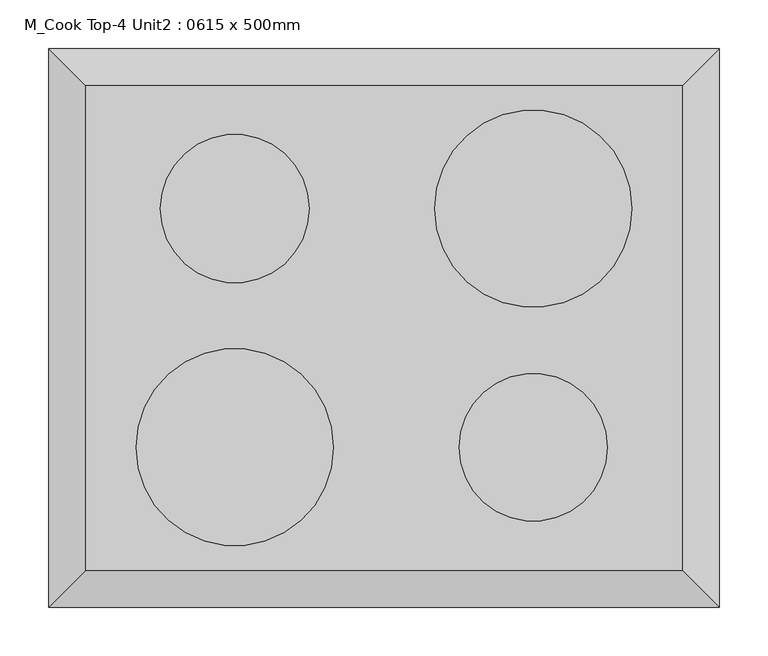
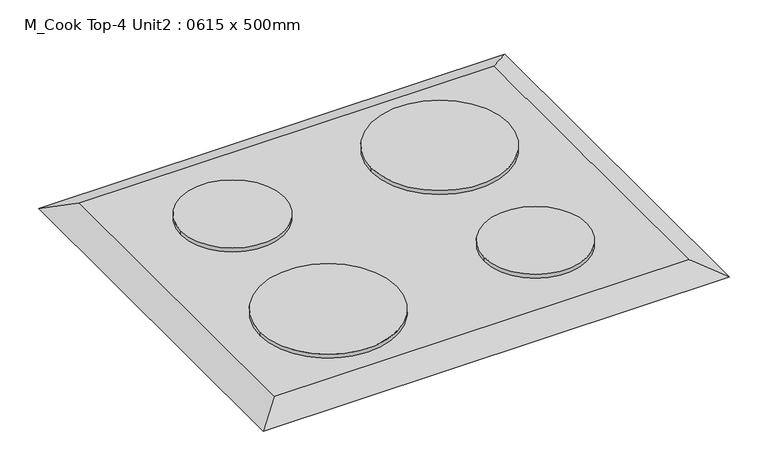
"""IFC4 building model written with IfcOpenShell, lengths in millimetres: proxy geometry, M_Cook Top-4 Unit2 : 0615 x 500mm."""

from ifc_helpers import new_model, si_unit, point, frame, frame_2d, origin, place, context, project, spatial, circle_curve, trimmed, segment, composite_curve, outline, extrude, faceted_brep, source, transform, mapped, element, save


def m_cook_top_4_unit2_0615_x_500mm_249f3515(model_context):
    return source(origin(), model_context, "Body", "SolidModel", [
        faceted_brep([(307.5, 250.0, 918.0), (-307.5, 250.0, 918.0), (-307.5, -250.0, 918.0), (307.5, -250.0, 918.0), (345.6, 288.1, 900.0), (345.6, -288.1, 900.0), (-345.6, -288.1, 900.0), (-345.6, 288.1, 900.0)], [[[0, 1, 2, 3]], [[4, 5, 6, 7]], [[4, 7, 1, 0]], [[7, 6, 2, 1]], [[6, 5, 3, 2]], [[5, 4, 0, 3]]]),
        extrude(outline(composite_curve([segment(trimmed(circle_curve(frame_2d((153.75, -123.0)), 76.2), [point((77.55, -123.0))], [point((229.95, -123.0))], False, "CARTESIAN"), True, "CONTINUOUS"), segment(trimmed(circle_curve(frame_2d((153.75, -123.0)), 76.2), [point((229.95, -123.0))], [point((77.55, -123.0))], False, "CARTESIAN"), True, "CONTINUOUS")], self_intersect=False)), frame((0.0, 0.0, 918.0), z_axis=(0.0, 0.0, 1.0), x_axis=(1.0, 0.0, 0.0)), (0.0, 0.0, 1.0), 6.35),
        extrude(outline(composite_curve([segment(trimmed(circle_curve(frame_2d((153.75, 123.0)), 101.6), [point((52.15, 123.0))], [point((255.35, 123.0))], False, "CARTESIAN"), True, "CONTINUOUS"), segment(trimmed(circle_curve(frame_2d((153.75, 123.0)), 101.6), [point((255.35, 123.0))], [point((52.15, 123.0))], False, "CARTESIAN"), True, "CONTINUOUS")], self_intersect=False)), frame((0.0, 0.0, 918.0), z_axis=(0.0, 0.0, 1.0), x_axis=(1.0, 0.0, 0.0)), (0.0, 0.0, 1.0), 6.35),
        extrude(outline(composite_curve([segment(trimmed(circle_curve(frame_2d((-153.75, 123.0)), 76.59), [point((-230.34, 123.0))], [point((-77.16, 123.0))], False, "CARTESIAN"), True, "CONTINUOUS"), segment(trimmed(circle_curve(frame_2d((-153.75, 123.0)), 76.59), [point((-77.16, 123.0))], [point((-230.34, 123.0))], False, "CARTESIAN"), True, "CONTINUOUS")], self_intersect=False)), frame((0.0, 0.0, 918.0), z_axis=(0.0, 0.0, 1.0), x_axis=(1.0, 0.0, 0.0)), (0.0, 0.0, 1.0), 6.35),
        extrude(outline(composite_curve([segment(trimmed(circle_curve(frame_2d((-153.75, -123.0)), 101.6), [point((-52.15, -123.0))], [point((-255.35, -123.0))], False, "CARTESIAN"), True, "CONTINUOUS"), segment(trimmed(circle_curve(frame_2d((-153.75, -123.0)), 101.6), [point((-255.35, -123.0))], [point((-52.15, -123.0))], False, "CARTESIAN"), True, "CONTINUOUS")], self_intersect=False)), frame((0.0, 0.0, 918.0), z_axis=(0.0, 0.0, 1.0), x_axis=(1.0, 0.0, 0.0)), (0.0, 0.0, 1.0), 6.35),
    ])


if __name__ == "__main__":
    model = new_model("IFC4")
    model_context = context("Model", 3, world=origin())
    ifc_project = project(units=[si_unit("LENGTHUNIT", "METRE", prefix="MILLI")], contexts=[model_context])
    site = spatial("IfcSite", under=ifc_project)
    building = spatial("IfcBuilding", under=site)
    placement = place(None, origin())
    m_cook_top_4_unit2_0615_x_500mm_shape = m_cook_top_4_unit2_0615_x_500mm_249f3515(model_context)
    element("IfcBuildingElementProxy", 1, Name="M_Cook Top-4 Unit2 : 0615 x 500mm", ObjectType="M_Cook Top-4 Unit2 : 0615 x 500mm", at=placement, inside=building, context=model_context, shape_type="MappedRepresentation", body=[
        mapped(m_cook_top_4_unit2_0615_x_500mm_shape, transform((0.0, 0.0, 0.0), x_axis=(1.0, 0.0, 0.0), y_axis=(0.0, 1.0, 0.0), z_axis=(0.0, 0.0, 1.0))),
    ])
    save(model, "model.ifc")

# Revit data of these elements
# Type "M_Cook Top-4 Unit2 : 0615 x 500mm"
#   Depth = 500 mm
#   Width = 615 mm
#   Burner Material = Steel, Chrome Plated
#   Cooktop Material = Steel, Polished
#   Default Elevation = 0
#   Assembly Code = ""
# Element 1 (IfcBuildingElementProxy, "M_Cook Top-4 Unit2 : 0615 x 500mm")
#   Materials on its faces: "Steel, Polished", "Steel, Chrome Plated"
# Materials
#   "Steel, Chrome Plated": class "Metal", colour RGB 244 244 244, transparency 0, Description = "Chromiuim plated steel", Cost = 0
#   "Steel, Polished": class "Metal", colour RGB 57 57 57, transparency 0, Description = "Polished steel", Cost = 0
